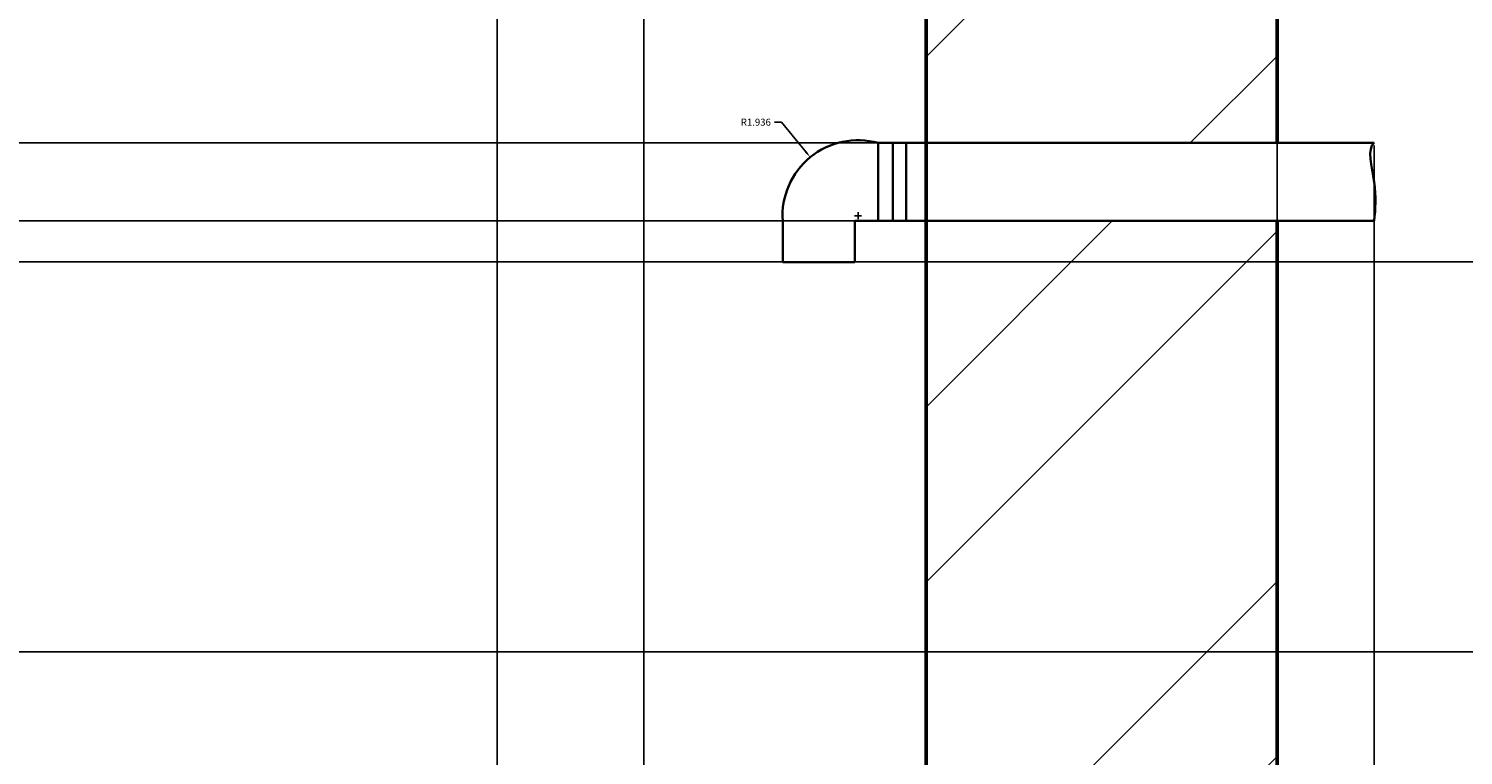
# Model space of a CAD drawing. Units: inches. Extents: x 2812 to 3051, y 1398 to 1659.
# Tile 21 of 65: x 2929 to 2966, y 1435 to 1453. Entities that reach past the tile are written whole.
import ezdxf

# ---------------------------------------------------------------- set-up
doc = ezdxf.new("R2010")
doc.units = ezdxf.units.IN
for name, color, linetype, lineweight in [('A-ANNO-DIMS', 2, 'Continuous', 18), ('P-SANR-PIPE', 4, 'Continuous', 35), ('S-CONC', 7, 'Continuous', 50), ('S-CONC-PATT', 8, 'Continuous', 18)]:
    doc.layers.add(name, color=color, linetype=linetype, lineweight=lineweight)
doc.styles.get("Standard").update_dxf_attribs({"font": 'arial.ttf'})
doc.dimstyles.get("Standard").update_dxf_attribs({"dimtxt": 0.18, "dimasz": 0.18, "dimexe": 0.18, "dimexo": 0.0625, "dimgap": 0.09, "dimtad": 0, "dimtih": 1, "dimtoh": 1, "dimdec": 4, "dimzin": 0, "dimdsep": 46, "dimtxsty": 'Standard', "dimcen": 0.09, "dimadec": 0, "dimazin": 0, "dimtfac": 1, "dimtdec": 4, "dimtofl": 0, "dimtmove": 0, "dimatfit": 3, "dimfxl": 1, "dimtolj": 1, "dimtzin": 0, "dimarcsym": 0})

# ---------------------------------------------------------------- blocks, each defined once
blk = doc.blocks.new('*D30')
at = {"layer": 'A-ANNO-DIMS', "color": 0, "lineweight": -2, "transparency": 16777216}
for p, q in [((2945.147, 1598.692), (2945.147, 1397.505)), ((2952.385, 1559.757), (2952.385, 1397.505)), ((2945.327, 1397.685), (2948.373, 1397.685)), ((2952.205, 1397.685), (2949.159, 1397.685))]:
    blk.add_line(p, q, dxfattribs=at)
at = {"layer": 'A-ANNO-DIMS', "color": 0, "transparency": 16777216}
for points in [[(2945.327, 1397.715), (2945.327, 1397.655), (2945.147, 1397.685)], [(2952.205, 1397.715), (2952.205, 1397.655), (2952.385, 1397.685)]]:
    blk.add_solid(points, dxfattribs=at)
at = {"layer": 'Defpoints', "color": 0, "transparency": 16777216}
for p in [(2945.147, 1598.754), (2952.385, 1559.82), (2952.385, 1397.685)]:
    blk.add_point(p, dxfattribs=at)
at = {"layer": 'A-ANNO-DIMS', "color": 0, "transparency": 16777216, "insert": (2948.766, 1397.685), "char_height": 0.18, "attachment_point": 5}
blk.add_mtext('\\A1;7.238', dxfattribs=at)
blk = doc.blocks.new('*D31')
at = {"layer": 'A-ANNO-DIMS', "color": 0, "lineweight": -2, "transparency": 16777216}
for p, q in [((2972.272, 1594.192), (2972.272, 1397.505)), ((2961.385, 1559.757), (2961.385, 1397.505)), ((2961.565, 1397.685), (2966.373, 1397.685)), ((2972.092, 1397.685), (2967.283, 1397.685))]:
    blk.add_line(p, q, dxfattribs=at)
at = {"layer": 'A-ANNO-DIMS', "color": 0, "transparency": 16777216}
for points in [[(2961.565, 1397.715), (2961.565, 1397.655), (2961.385, 1397.685)], [(2972.092, 1397.715), (2972.092, 1397.655), (2972.272, 1397.685)]]:
    blk.add_solid(points, dxfattribs=at)
at = {"layer": 'Defpoints', "color": 0, "transparency": 16777216}
for p in [(2972.272, 1594.254), (2961.385, 1559.82), (2972.272, 1397.685)]:
    blk.add_point(p, dxfattribs=at)
at = {"layer": 'A-ANNO-DIMS', "color": 0, "transparency": 16777216, "insert": (2966.828, 1397.685), "char_height": 0.18, "attachment_point": 5}
blk.add_mtext('\\A1;10.887', dxfattribs=at)
blk = doc.blocks.new('*D45')
at = {"layer": 'A-ANNO-DIMS', "color": 0, "lineweight": -2, "transparency": 16777216}
for p, q in [((2896.385, 1487.973), (2896.385, 1397.505)), ((2941.385, 1487.973), (2941.385, 1397.505)), ((2896.565, 1397.685), (2918.662, 1397.685)), ((2941.205, 1397.685), (2919.108, 1397.685))]:
    blk.add_line(p, q, dxfattribs=at)
at = {"layer": 'A-ANNO-DIMS', "color": 0, "transparency": 16777216}
for points in [[(2896.565, 1397.715), (2896.565, 1397.655), (2896.385, 1397.685)], [(2941.205, 1397.715), (2941.205, 1397.655), (2941.385, 1397.685)]]:
    blk.add_solid(points, dxfattribs=at)
at = {"layer": 'Defpoints', "color": 0, "transparency": 16777216}
for p in [(2896.385, 1488.035), (2941.385, 1488.035), (2941.385, 1397.685)]:
    blk.add_point(p, dxfattribs=at)
at = {"layer": 'A-ANNO-DIMS', "color": 0, "transparency": 16777216, "insert": (2918.885, 1397.685), "char_height": 0.18, "attachment_point": 5}
blk.add_mtext('\\A1;45', dxfattribs=at)
blk = doc.blocks.new('*D46')
at = {"layer": 'A-ANNO-DIMS', "color": 0, "lineweight": -2, "transparency": 16777216}
for p, q in [((2941.385, 1487.973), (2941.385, 1397.505)), ((2970.385, 1487.973), (2970.385, 1397.505)), ((2941.565, 1397.685), (2955.664, 1397.685)), ((2970.205, 1397.685), (2956.106, 1397.685))]:
    blk.add_line(p, q, dxfattribs=at)
at = {"layer": 'A-ANNO-DIMS', "color": 0, "transparency": 16777216}
for points in [[(2941.565, 1397.715), (2941.565, 1397.655), (2941.385, 1397.685)], [(2970.205, 1397.715), (2970.205, 1397.655), (2970.385, 1397.685)]]:
    blk.add_solid(points, dxfattribs=at)
at = {"layer": 'Defpoints', "color": 0, "transparency": 16777216}
for p in [(2941.385, 1488.035), (2970.385, 1488.035), (2970.385, 1397.685)]:
    blk.add_point(p, dxfattribs=at)
at = {"layer": 'A-ANNO-DIMS', "color": 0, "transparency": 16777216, "insert": (2955.885, 1397.685), "char_height": 0.18, "attachment_point": 5}
blk.add_mtext('\\A1;29', dxfattribs=at)
blk = doc.blocks.new('*D56')
at = {"layer": 'A-ANNO-DIMS', "color": 0, "lineweight": -2, "transparency": 16777216}
for p, q in [((2880.322, 1452.035), (2811.806, 1452.035)), ((2811.986, 1451.855), (2811.986, 1434.217)), ((2811.986, 1416.215), (2811.986, 1433.853)), ((2952.322, 1416.035), (2811.806, 1416.035))]:
    blk.add_line(p, q, dxfattribs=at)
at = {"layer": 'A-ANNO-DIMS', "color": 0, "transparency": 16777216}
for points in [[(2811.956, 1451.855), (2812.016, 1451.855), (2811.986, 1452.035)], [(2811.956, 1416.215), (2812.016, 1416.215), (2811.986, 1416.035)]]:
    blk.add_solid(points, dxfattribs=at)
at = {"layer": 'Defpoints', "color": 0, "transparency": 16777216}
for p in [(2811.986, 1452.035), (2880.385, 1452.035), (2952.385, 1416.035)]:
    blk.add_point(p, dxfattribs=at)
at = {"layer": 'A-ANNO-DIMS', "color": 0, "transparency": 16777216, "insert": (2811.986, 1434.035), "char_height": 0.18, "attachment_point": 5}
blk.add_mtext('\\A1;36', dxfattribs=at)
blk = doc.blocks.new('*D65')
at = {"layer": 'A-ANNO-DIMS', "color": 0, "lineweight": -2, "transparency": 16777216}
for p, q in [((2920.62, 1437.426), (3051.178, 1437.426)), ((3050.998, 1437.246), (3050.998, 1432.608)), ((3050.998, 1427.606), (3050.998, 1432.245)), ((2929.438, 1427.426), (3051.178, 1427.426))]:
    blk.add_line(p, q, dxfattribs=at)
at = {"layer": 'A-ANNO-DIMS', "color": 0, "transparency": 16777216}
for points in [[(3050.968, 1437.246), (3051.028, 1437.246), (3050.998, 1437.426)], [(3050.968, 1427.606), (3051.028, 1427.606), (3050.998, 1427.426)]]:
    blk.add_solid(points, dxfattribs=at)
at = {"layer": 'Defpoints', "color": 0, "transparency": 16777216}
for p in [(2920.558, 1437.426), (3050.998, 1437.426), (2929.375, 1427.426)]:
    blk.add_point(p, dxfattribs=at)
at = {"layer": 'A-ANNO-DIMS', "color": 0, "transparency": 16777216, "insert": (3050.998, 1432.426), "char_height": 0.18, "attachment_point": 5}
blk.add_mtext('\\A1;10', dxfattribs=at)
blk = doc.blocks.new('*D66')
at = {"layer": 'A-ANNO-DIMS', "color": 0, "lineweight": -2, "transparency": 16777216}
for p, q in [((2914.018, 1447.426), (3051.178, 1447.426)), ((3050.998, 1447.246), (3050.998, 1442.608)), ((3050.998, 1437.606), (3050.998, 1442.245)), ((2920.62, 1437.426), (3051.178, 1437.426))]:
    blk.add_line(p, q, dxfattribs=at)
at = {"layer": 'A-ANNO-DIMS', "color": 0, "transparency": 16777216}
for points in [[(3050.968, 1447.246), (3051.028, 1447.246), (3050.998, 1447.426)], [(3050.968, 1437.606), (3051.028, 1437.606), (3050.998, 1437.426)]]:
    blk.add_solid(points, dxfattribs=at)
at = {"layer": 'Defpoints', "color": 0, "transparency": 16777216}
for p in [(2913.955, 1447.426), (3050.998, 1447.426), (2920.558, 1437.426)]:
    blk.add_point(p, dxfattribs=at)
at = {"layer": 'A-ANNO-DIMS', "color": 0, "transparency": 16777216, "insert": (3050.998, 1442.426), "char_height": 0.18, "attachment_point": 5}
blk.add_mtext('\\A1;10', dxfattribs=at)
blk = doc.blocks.new('*D67')
at = {"layer": 'A-ANNO-DIMS', "color": 0, "lineweight": -2, "transparency": 16777216}
for p, q in [((2906.065, 1457.426), (3051.178, 1457.426)), ((3050.998, 1457.246), (3050.998, 1452.608)), ((3050.998, 1447.606), (3050.998, 1452.245)), ((2914.018, 1447.426), (3051.178, 1447.426))]:
    blk.add_line(p, q, dxfattribs=at)
at = {"layer": 'A-ANNO-DIMS', "color": 0, "transparency": 16777216}
for points in [[(3050.968, 1457.246), (3051.028, 1457.246), (3050.998, 1457.426)], [(3050.968, 1447.606), (3051.028, 1447.606), (3050.998, 1447.426)]]:
    blk.add_solid(points, dxfattribs=at)
at = {"layer": 'Defpoints', "color": 0, "transparency": 16777216}
for p in [(2906.002, 1457.426), (3050.998, 1457.426), (2913.955, 1447.426)]:
    blk.add_point(p, dxfattribs=at)
at = {"layer": 'A-ANNO-DIMS', "color": 0, "transparency": 16777216, "insert": (3050.998, 1452.426), "char_height": 0.18, "attachment_point": 5}
blk.add_mtext('\\A1;10', dxfattribs=at)
blk = doc.blocks.new('*D70')
at = {"layer": 'A-ANNO-DIMS', "color": 0, "lineweight": -2, "transparency": 16777216}
for p, q in [((2961.385, 1450.411), (2961.385, 1397.505)), ((2963.874, 1450.411), (2963.874, 1397.505)), ((2961.565, 1397.685), (2962.234, 1397.685)), ((2963.694, 1397.685), (2963.025, 1397.685))]:
    blk.add_line(p, q, dxfattribs=at)
at = {"layer": 'A-ANNO-DIMS', "color": 0, "transparency": 16777216}
for points in [[(2961.565, 1397.715), (2961.565, 1397.655), (2961.385, 1397.685)], [(2963.694, 1397.715), (2963.694, 1397.655), (2963.874, 1397.685)]]:
    blk.add_solid(points, dxfattribs=at)
at = {"layer": 'Defpoints', "color": 0, "transparency": 16777216}
for p in [(2961.385, 1450.474), (2963.874, 1450.474), (2963.874, 1397.685)]:
    blk.add_point(p, dxfattribs=at)
at = {"layer": 'A-ANNO-DIMS', "color": 0, "transparency": 16777216, "insert": (2962.63, 1397.685), "char_height": 0.18, "attachment_point": 5}
blk.add_mtext('\\A1;2.489', dxfattribs=at)
blk = doc.blocks.new('*D75')
at = {"layer": 'A-ANNO-DIMS', "color": 0, "lineweight": -2, "transparency": 16777216}
for p, q in [((2963.812, 1448.474), (2811.806, 1448.474)), ((2811.986, 1448.294), (2811.986, 1432.437)), ((2811.986, 1416.215), (2811.986, 1432.073)), ((2961.322, 1416.035), (2811.806, 1416.035))]:
    blk.add_line(p, q, dxfattribs=at)
at = {"layer": 'A-ANNO-DIMS', "color": 0, "transparency": 16777216}
for points in [[(2811.956, 1448.294), (2812.016, 1448.294), (2811.986, 1448.474)], [(2811.956, 1416.215), (2812.016, 1416.215), (2811.986, 1416.035)]]:
    blk.add_solid(points, dxfattribs=at)
at = {"layer": 'Defpoints', "color": 0, "transparency": 16777216}
for p in [(2811.986, 1448.474), (2963.874, 1448.474), (2961.385, 1416.035)]:
    blk.add_point(p, dxfattribs=at)
at = {"layer": 'A-ANNO-DIMS', "color": 0, "transparency": 16777216, "insert": (2811.986, 1432.255), "char_height": 0.18, "attachment_point": 5}
blk.add_mtext('\\A1;32.44', dxfattribs=at)
blk = doc.blocks.new('*D76')
at = {"layer": 'A-ANNO-DIMS', "color": 0, "lineweight": -2, "transparency": 16777216}
for p, q in [((2963.812, 1450.474), (2811.806, 1450.474)), ((2811.986, 1450.294), (2811.986, 1449.654)), ((2811.986, 1448.654), (2811.986, 1449.293)), ((2963.812, 1448.474), (2811.806, 1448.474))]:
    blk.add_line(p, q, dxfattribs=at)
at = {"layer": 'A-ANNO-DIMS', "color": 0, "transparency": 16777216}
for points in [[(2811.956, 1450.294), (2812.016, 1450.294), (2811.986, 1450.474)], [(2811.956, 1448.654), (2812.016, 1448.654), (2811.986, 1448.474)]]:
    blk.add_solid(points, dxfattribs=at)
at = {"layer": 'Defpoints', "color": 0, "transparency": 16777216}
for p in [(2811.986, 1450.474), (2963.874, 1450.474), (2963.874, 1448.474)]:
    blk.add_point(p, dxfattribs=at)
at = {"layer": 'A-ANNO-DIMS', "color": 0, "transparency": 16777216, "insert": (2811.986, 1449.474), "char_height": 0.18, "attachment_point": 5}
blk.add_mtext('\\A1;2', dxfattribs=at)
blk = doc.blocks.new('*D77')
at = {"layer": 'A-ANNO-DIMS', "color": 0, "lineweight": -2, "transparency": 16777216}
for p, q in [((2961.322, 1472.035), (2811.806, 1472.035)), ((2811.986, 1471.855), (2811.986, 1461.436)), ((2811.986, 1450.654), (2811.986, 1461.073)), ((2963.812, 1450.474), (2811.806, 1450.474))]:
    blk.add_line(p, q, dxfattribs=at)
at = {"layer": 'A-ANNO-DIMS', "color": 0, "transparency": 16777216}
for points in [[(2811.956, 1471.855), (2812.016, 1471.855), (2811.986, 1472.035)], [(2811.956, 1450.654), (2812.016, 1450.654), (2811.986, 1450.474)]]:
    blk.add_solid(points, dxfattribs=at)
at = {"layer": 'Defpoints', "color": 0, "transparency": 16777216}
for p in [(2811.986, 1472.035), (2961.385, 1472.035), (2963.874, 1450.474)]:
    blk.add_point(p, dxfattribs=at)
at = {"layer": 'A-ANNO-DIMS', "color": 0, "transparency": 16777216, "insert": (2811.986, 1461.255), "char_height": 0.18, "attachment_point": 5}
blk.add_mtext('\\A1;21.56', dxfattribs=at)
blk = doc.blocks.new('*D86')
at = {"layer": 'A-ANNO-DIMS', "color": 0, "lineweight": -2, "transparency": 16777216}
for p, q in [((2948.498, 1451.006), (2948.678, 1451.006)), ((2948.678, 1451.006), (2949.3, 1450.246)), ((2950.549, 1448.607), (2950.729, 1448.607)), ((2950.639, 1448.517), (2950.639, 1448.697))]:
    blk.add_line(p, q, dxfattribs=at)
at = {"layer": 'A-ANNO-DIMS', "color": 0, "transparency": 16777216}
blk.add_solid([(2949.323, 1450.265), (2949.277, 1450.227), (2949.414, 1450.106)], dxfattribs=at)
at = {"layer": 'Defpoints', "color": 0, "transparency": 16777216}
for p in [(2949.414, 1450.106), (2950.639, 1448.607)]:
    blk.add_point(p, dxfattribs=at)
at = {"layer": 'A-ANNO-DIMS', "color": 0, "transparency": 16777216, "insert": (2948.019, 1451.006), "char_height": 0.18, "attachment_point": 5}
blk.add_mtext('\\A1;R1.936', dxfattribs=at)

msp = doc.modelspace()

# ---------------------------------------------------------------- hatches: boundary and pattern name
at = {"layer": 'S-CONC-PATT'}
h = msp.add_hatch(dxfattribs=at)
h.set_pattern_fill('ANSI32', color=256)
h.paths.add_polyline_path([(3027.3849, 1646.82), (2835.3849, 1646.82), (2835.3849, 1603.2296), (2844.3849, 1603.2296), (2844.3849, 1637.82), (3018.3849, 1637.82), (3018.3849, 1602.5441), (3027.3849, 1602.5441)])
h.paths.add_polyline_path([(2844.3849, 1594.2296), (2835.3849, 1594.2296), (2835.3849, 1550.82), (3027.3849, 1550.82), (3027.3849, 1593.5441), (3018.3849, 1593.5441), (3018.3849, 1559.82), (2844.3849, 1559.82)])
h.paths.add_polyline_path([(2844.3849, 1482.0354), (2835.3849, 1482.0354), (2835.3849, 1463.4959), (2844.3849, 1463.4959)])
h.paths.add_polyline_path([(2844.3849, 1461.4959), (2835.3849, 1461.4959), (2835.3849, 1416.0354), (2844.3849, 1416.0354)])
h.paths.add_polyline_path([(3027.3849, 1482.0354), (3018.3849, 1482.0354), (3018.3849, 1463.2854), (3027.3849, 1463.2854)])
h.paths.add_polyline_path([(3027.3849, 1461.2854), (3018.3849, 1461.2854), (3018.3849, 1416.0354), (3027.3849, 1416.0354)])
h.paths.add_polyline_path([(2961.3849, 1448.4738), (2952.3849, 1448.4738), (2952.3849, 1416.0354), (2961.3849, 1416.0354)])
h.paths.add_polyline_path([(2961.3849, 1462.3026), (2952.3849, 1462.3026), (2952.3849, 1450.4738), (2961.3849, 1450.4738)])
h.paths.add_polyline_path([(2961.3849, 1472.0354), (2952.3849, 1472.0354), (2952.3849, 1462.3026), (2961.3849, 1462.3026)])

# ---------------------------------------------------------------- linework, layer by layer
at = {"layer": 'P-SANR-PIPE'}
for p, q in [((2951.8741, 1450.4738), (2951.1541, 1450.4738)), ((2951.1541, 1448.4738), (2951.1541, 1450.4738)), ((2951.5327, 1450.4738), (2951.5327, 1448.4738)), ((2951.8741, 1448.4738), (2951.8741, 1450.4738)), ((2951.8741, 1450.4738), (2963.8741, 1450.4738)), ((2951.8741, 1450.4738), (2952.3741, 1450.4738)), ((2952.3741, 1450.4738), (2952.3741, 1448.4738)), ((2948.7077, 1447.4185), (2948.7077, 1448.4738)), ((2951.1541, 1448.4738), (2950.5541, 1448.4738)), ((2950.5541, 1448.4738), (2950.5541, 1447.4185)), ((2951.5327, 1448.4738), (2951.1541, 1448.4738)), ((2963.8741, 1448.4738), (2951.5327, 1448.4738)), ((2950.5541, 1447.4185), (2948.7077, 1447.4185))]:
    msp.add_line(p, q, dxfattribs=at)
msp.add_arc((2950.6391, 1448.6074), 1.9361, 74.57374, 183.95951, dxfattribs=at)
msp.add_open_spline([(2963.8741, 1448.4738), (2963.9023, 1448.7789), (2963.9585, 1449.3893), (2963.6771, 1450.3374), (2963.8741, 1450.4738)], degree=3, dxfattribs=at)
at = {"layer": 'S-CONC'}
for p, q in [((2952.3849, 1472.0354), (2952.3849, 1416.0354)), ((2961.3849, 1472.0354), (2961.3849, 1450.4738)), ((2961.3849, 1448.4738), (2961.3849, 1416.0354))]:
    msp.add_line(p, q, dxfattribs=at)

# ---------------------------------------------------------------- dimensions: what is measured, and where the dimension line sits
at = {"layer": 'A-ANNO-DIMS'}
for base, p1, p2, override, picture, middle in [((2952.3849, 1397.6854), (2945.1467, 1598.7541), (2952.3849, 1559.82), {"dimdec": 3, "dimlfac": 1, "dimrnd": 0, "dimzin": 0, "dimdsep": 46, "dimlunit": 2}, '*D30', (2948.7658, 1397.6854)), ((2972.2716, 1397.6854), (2961.3849, 1559.82), (2972.2716, 1594.2541), {"dimdec": 3, "dimlfac": 1, "dimrnd": 0, "dimzin": 0, "dimdsep": 46, "dimlunit": 2}, '*D31', (2966.8282, 1397.6854)), ((2941.3849, 1397.6854), (2896.3849, 1488.0354), (2941.3849, 1488.0354), {"dimdec": 0, "dimlfac": 1, "dimrnd": 0, "dimzin": 0, "dimdsep": 46, "dimlunit": 2}, '*D45', (2918.8849, 1397.6854)), ((2970.3849, 1397.6854), (2941.3849, 1488.0354), (2970.3849, 1488.0354), {"dimdec": 0, "dimlfac": 1, "dimrnd": 0, "dimzin": 0, "dimdsep": 46, "dimlunit": 2}, '*D46', (2955.8849, 1397.6854)), ((2963.8741, 1397.6854), (2961.3849, 1450.4738), (2963.8741, 1450.4738), {"dimdec": 3, "dimlfac": 1, "dimrnd": 0, "dimzin": 0, "dimdsep": 46, "dimlunit": 2}, '*D70', (2962.6295, 1397.6854))]:
    dim = msp.add_linear_dim(base=base, p1=p1, p2=p2, dimstyle='Standard', override=override, dxfattribs=at)
    dim.commit()
    dim.dimension.update_dxf_attribs({"geometry": picture, "text_midpoint": middle})
for base, p1, p2, override, picture, middle in [((2811.9855, 1472.0354), (2963.8741, 1450.4738), (2961.3849, 1472.0354), {"dimdec": 2, "dimlfac": 1, "dimrnd": 0, "dimzin": 0, "dimdsep": 46, "dimlunit": 2}, '*D77', (2811.9855, 1461.2546)), ((3050.998, 1457.4265), (2913.9551, 1447.4265), (2906.0021, 1457.4265), {"dimdec": 0, "dimlfac": 1, "dimrnd": 0, "dimzin": 0, "dimdsep": 46, "dimlunit": 2}, '*D67', (3050.998, 1452.4265)), ((2811.9855, 1452.0354), (2952.3849, 1416.0354), (2880.3849, 1452.0354), {"dimdec": 0, "dimlfac": 1, "dimrnd": 0, "dimzin": 0, "dimdsep": 46, "dimlunit": 2}, '*D56', (2811.9855, 1434.0354)), ((2811.9855, 1450.4738), (2963.8741, 1448.4738), (2963.8741, 1450.4738), {"dimdec": 0, "dimlfac": 1, "dimrnd": 0, "dimzin": 0, "dimdsep": 46, "dimlunit": 2}, '*D76', (2811.9855, 1449.4738)), ((2811.9855, 1448.4738), (2961.3849, 1416.0354), (2963.8741, 1448.4738), {"dimdec": 2, "dimlfac": 1, "dimrnd": 0, "dimzin": 0, "dimdsep": 46, "dimlunit": 2}, '*D75', (2811.9855, 1432.2546)), ((3050.998, 1447.4265), (2920.5577, 1437.4265), (2913.9551, 1447.4265), {"dimdec": 0, "dimlfac": 1, "dimrnd": 0, "dimzin": 0, "dimdsep": 46, "dimlunit": 2}, '*D66', (3050.998, 1442.4265)), ((3050.998, 1437.4265), (2929.3751, 1427.4265), (2920.5577, 1437.4265), {"dimdec": 0, "dimlfac": 1, "dimrnd": 0, "dimzin": 0, "dimdsep": 46, "dimlunit": 2}, '*D65', (3050.998, 1432.4265))]:
    dim = msp.add_linear_dim(base=base, p1=p1, p2=p2, angle=90, dimstyle='Standard', override=override, dxfattribs=at)
    dim.commit()
    dim.dimension.update_dxf_attribs({"geometry": picture, "text_midpoint": middle})
dim = msp.add_radius_dim(center=(2950.6391, 1448.6074), mpoint=(2949.4137, 1450.1063), dimstyle='Standard', override={"dimdec": 3, "dimlfac": 1, "dimrnd": 0, "dimzin": 0, "dimdsep": 46, "dimlunit": 2}, dxfattribs=at)
dim.commit()
dim.dimension.update_dxf_attribs({"geometry": '*D86', "text_midpoint": (2948.0187, 1451.0057), "dimtype": 164})

doc.saveas('drawing.dxf')
